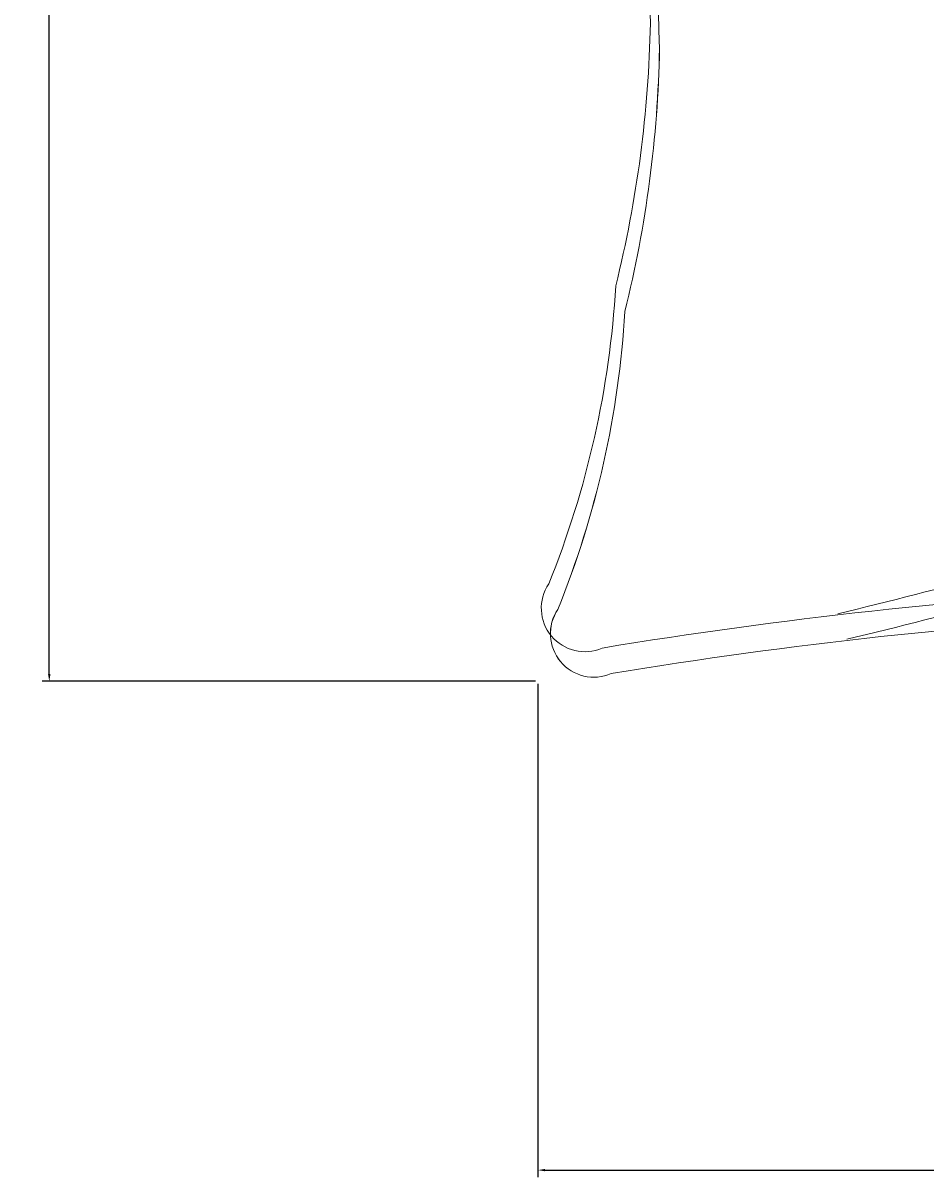
# Model space of a CAD drawing. Units: inches. Extents: x 1885 to 2748, y 783 to 2421.
# Tile 92 of 117: x 2372 to 2395, y 2253 to 2282. Entities that reach past the tile are written whole.
import ezdxf

# ---------------------------------------------------------------- set-up
doc = ezdxf.new("R2010")
doc.units = ezdxf.units.IN
doc.layers.add('A-ANNO-DIMS', color=2, linetype='Continuous', lineweight=18)
doc.layers.add('A-FURN', color=8, linetype='Continuous', lineweight=13)
doc.styles.get("Standard").update_dxf_attribs({"font": 'arial.ttf'})
doc.dimstyles.get("Standard").update_dxf_attribs({"dimtxt": 0.18, "dimasz": 0.18, "dimexe": 0.18, "dimexo": 0.0625, "dimgap": 0.09, "dimtad": 0, "dimtih": 1, "dimtoh": 1, "dimdec": 4, "dimzin": 0, "dimdsep": 46, "dimtxsty": 'Standard', "dimcen": 0.09, "dimadec": 0, "dimazin": 0, "dimtfac": 1, "dimtdec": 4, "dimtofl": 0, "dimtmove": 0, "dimatfit": 3, "dimfxl": 1, "dimtolj": 1, "dimtzin": 0, "dimarcsym": 0})

# ---------------------------------------------------------------- blocks, each defined once
blk = doc.blocks.new('BED-DOUBLE')
for centre, radius, start, end in [((-23.069, -16.995), 106.459, 13.38322, 17.70533), ((-23.069, -16.995), 106.459, 13.38322, 17.70533), ((-23.708, -17.223), 106.459, 13.38322, 17.70533), ((-23.708, -17.223), 106.459, 13.38322, 17.70533), ((201.48, 21.654), 121.759, 182.99578, 189.40907), ((201.48, 21.654), 121.759, 182.99578, 189.40907), ((200.841, 21.425), 121.759, 182.99578, 189.40907), ((200.841, 21.425), 121.759, 182.99578, 189.40907), ((51.257, 485.049), 482.31, 268.22771, 271.71854), ((51.257, 485.049), 482.31, 268.22771, 271.71854), ((65.158, -26.672), 29.634, 76.0648, 88.9113), ((65.158, -26.673), 29.634, 76.0648, 88.9113), ((50.617, 484.821), 482.31, 268.22771, 271.71854), ((64.519, -26.901), 29.634, 76.0648, 88.9113), ((64.519, -26.901), 29.634, 76.0648, 88.9113), ((70.919, -21.432), 23.562, 67.9751, 86.652), ((70.919, -21.433), 23.562, 67.9751, 86.652), ((70.279, -21.661), 23.562, 67.9751, 86.652), ((70.279, -21.661), 23.562, 67.9751, 86.652), ((80.361, 1.315), 1.089, 236.1736, 23.4781), ((80.361, 1.314), 1.089, 236.1736, 23.4781), ((79.721, 1.086), 1.089, 236.1736, 23.4781), ((79.721, 1.086), 1.089, 236.1736, 23.4781)]:
    blk.add_arc(centre, radius, start, end)
blk = doc.blocks.new('*D27')
at = {"layer": 'A-ANNO-DIMS', "color": 0, "lineweight": -2, "transparency": 16777216}
for p, q in [((2385.079, 2346.649), (2372.729, 2346.649)), ((2372.909, 2346.469), (2372.909, 2306.056)), ((2372.909, 2265.28), (2372.909, 2305.693)), ((2385.079, 2265.1), (2372.729, 2265.1))]:
    blk.add_line(p, q, dxfattribs=at)
at = {"layer": 'A-ANNO-DIMS', "color": 0, "transparency": 16777216}
for points in [[(2372.879, 2346.469), (2372.939, 2346.469), (2372.909, 2346.649)], [(2372.879, 2265.28), (2372.939, 2265.28), (2372.909, 2265.1)]]:
    blk.add_solid(points, dxfattribs=at)
at = {"layer": 'Defpoints', "color": 0, "transparency": 16777216}
for p in [(2385.141, 2346.649), (2372.909, 2265.1), (2385.141, 2265.1)]:
    blk.add_point(p, dxfattribs=at)
at = {"layer": 'A-ANNO-DIMS', "color": 0, "transparency": 16777216, "insert": (2372.909, 2305.874), "char_height": 0.18, "attachment_point": 5}
blk.add_mtext('\\A1;BED 82 TYP.', dxfattribs=at)
blk = doc.blocks.new('*D28')
at = {"layer": 'A-ANNO-DIMS', "color": 0, "lineweight": -2, "transparency": 16777216}
for p, q in [((2385.141, 2265.038), (2385.141, 2252.688)), ((2440.966, 2265.038), (2440.966, 2252.688)), ((2385.321, 2252.868), (2412.525, 2252.868)), ((2440.786, 2252.868), (2413.581, 2252.868))]:
    blk.add_line(p, q, dxfattribs=at)
at = {"layer": 'A-ANNO-DIMS', "color": 0, "transparency": 16777216}
for points in [[(2385.321, 2252.898), (2385.321, 2252.838), (2385.141, 2252.868)], [(2440.786, 2252.898), (2440.786, 2252.838), (2440.966, 2252.868)]]:
    blk.add_solid(points, dxfattribs=at)
at = {"layer": 'Defpoints', "color": 0, "transparency": 16777216}
for p in [(2385.141, 2265.1), (2440.966, 2265.1), (2440.966, 2252.868)]:
    blk.add_point(p, dxfattribs=at)
at = {"layer": 'A-ANNO-DIMS', "color": 0, "transparency": 16777216, "insert": (2413.053, 2252.868), "char_height": 0.18, "attachment_point": 5}
blk.add_mtext('\\A1;56 TYP.', dxfattribs=at)

msp = doc.modelspace()

# ---------------------------------------------------------------- block references
at = {"layer": 'A-FURN', "rotation": 269.9999998331857}
msp.add_blockref('BED-DOUBLE', (2385.229, 2346.652), dxfattribs=at)

# ---------------------------------------------------------------- dimensions: what is measured, and where the dimension line sits
at = {"layer": 'A-ANNO-DIMS'}
for base, p1, p2, angle, text, picture, middle in [((2372.909, 2265.1), (2385.141, 2346.649), (2385.141, 2265.1), 270, 'BED <> TYP.', '*D27', (2372.909, 2305.874)), ((2440.966, 2252.868), (2385.141, 2265.1), (2440.966, 2265.1), 360, '<> TYP.', '*D28', (2413.053, 2252.868))]:
    dim = msp.add_linear_dim(base=base, p1=p1, p2=p2, angle=angle, text=text, dimstyle='Standard', override={"dimdec": 0, "dimlfac": 1, "dimrnd": 0, "dimzin": 0, "dimdsep": 46, "dimlunit": 2}, dxfattribs=at)
    dim.commit()
    dim.dimension.update_dxf_attribs({"geometry": picture, "text_midpoint": middle})

doc.saveas('drawing.dxf')
